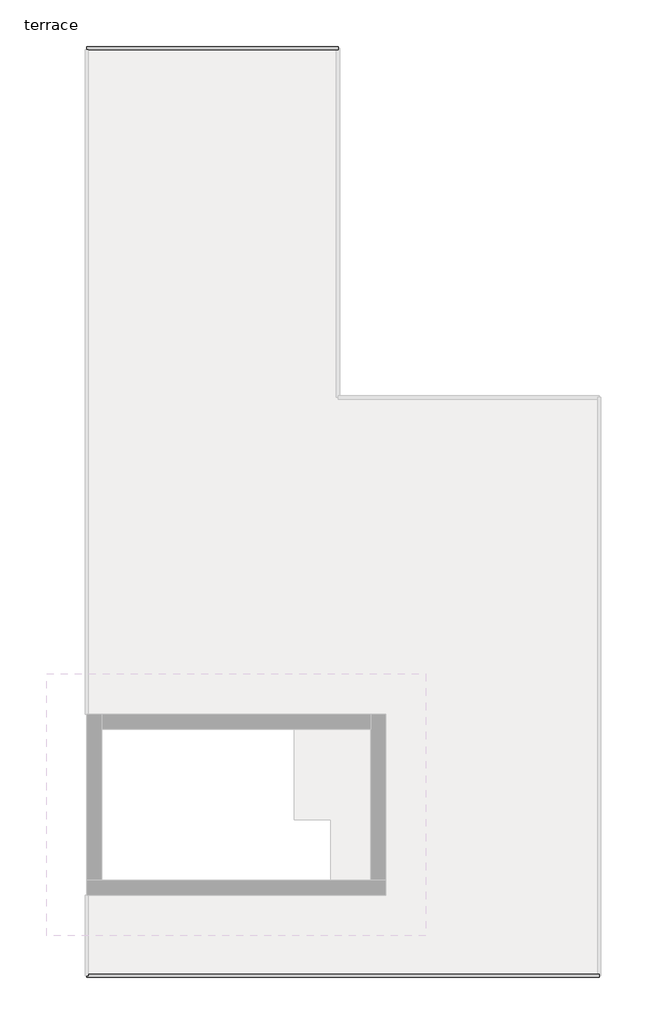
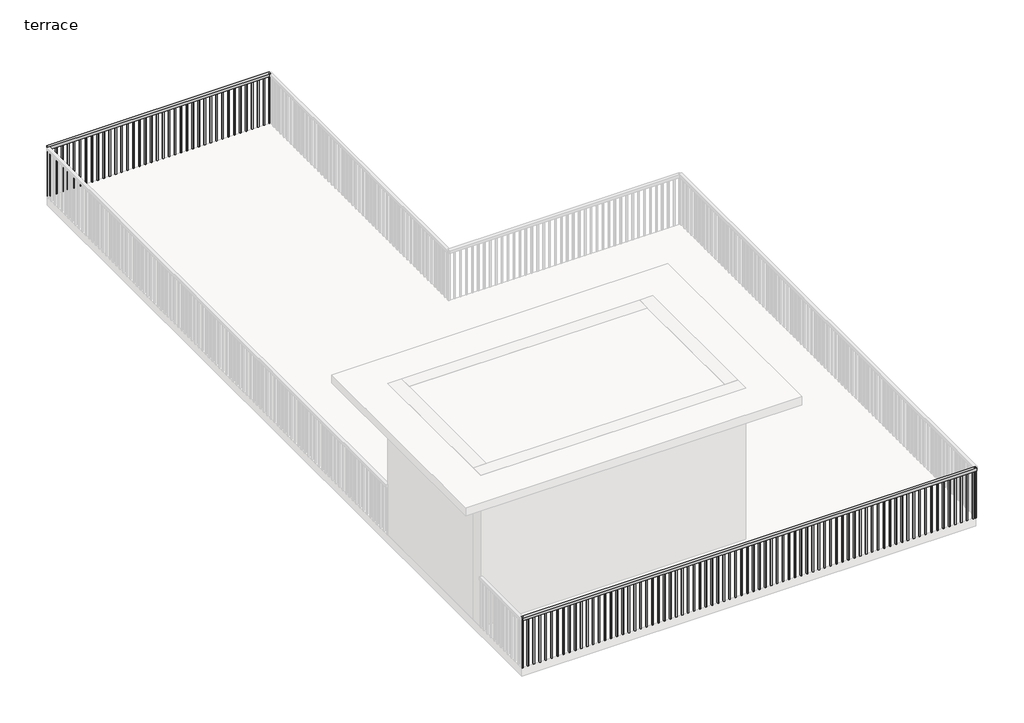
# One storey, part 2 of 4: 2 railings.
"""IFC4 building model written with IfcOpenShell, lengths in millimetres."""

from ifc_helpers import new_model, si_unit, frame, origin, place, context, project, spatial, polyline, outline, extrude, element, save

model = new_model("IFC4")

# Units and contexts
model_context = context("Model", 3, world=origin())
ifc_project = project(units=[si_unit("LENGTHUNIT", "METRE", prefix="MILLI")], contexts=[model_context])

# Site, building, storey
site = spatial("IfcSite", under=ifc_project)
building = spatial("IfcBuilding", under=site)
storey = spatial("IfcBuildingStorey", under=building, Name="terrace", Elevation=7010.4)

# Railings
placement = place(None, origin())
element("IfcRailing", 1, ObjectType="Handrail - Rectangular", at=placement, inside=storey, context=model_context, shape_type="SweptSolid", body=[
    extrude(outline(polyline([(32192.3316163, 19683.6980552), (32192.3316163, 19632.8980552), (28382.3316163, 19632.8980552), (28382.3316163, 19683.6980552), (32192.3316163, 19683.6980552)])), frame((0.0, 0.0, 7874.0), z_axis=(0.0, 0.0, 1.0), x_axis=(1.0, 0.0, 0.0)), (0.0, 0.0, 1.0), 50.8),
    extrude(outline(polyline([(28442.6566163, 19667.8230552), (28442.6566163, 19648.7730552), (28423.6066163, 19648.7730552), (28423.6066163, 19667.8230552), (28442.6566163, 19667.8230552)])), frame((0.0, 0.0, 7010.4), z_axis=(0.0, 0.0, 1.0), x_axis=(1.0, 0.0, 0.0)), (0.0, 0.0, 1.0), 863.6),
    extrude(outline(polyline([(28544.2566163, 19667.8230552), (28544.2566163, 19648.7730552), (28525.2066163, 19648.7730552), (28525.2066163, 19667.8230552), (28544.2566163, 19667.8230552)])), frame((0.0, 0.0, 7010.4), z_axis=(0.0, 0.0, 1.0), x_axis=(1.0, 0.0, 0.0)), (0.0, 0.0, 1.0), 863.6),
    extrude(outline(polyline([(28645.8566163, 19667.8230552), (28645.8566163, 19648.7730552), (28626.8066163, 19648.7730552), (28626.8066163, 19667.8230552), (28645.8566163, 19667.8230552)])), frame((0.0, 0.0, 7010.4), z_axis=(0.0, 0.0, 1.0), x_axis=(1.0, 0.0, 0.0)), (0.0, 0.0, 1.0), 863.6),
    extrude(outline(polyline([(28747.4566163, 19667.8230552), (28747.4566163, 19648.7730552), (28728.4066163, 19648.7730552), (28728.4066163, 19667.8230552), (28747.4566163, 19667.8230552)])), frame((0.0, 0.0, 7010.4), z_axis=(0.0, 0.0, 1.0), x_axis=(1.0, 0.0, 0.0)), (0.0, 0.0, 1.0), 863.6),
    extrude(outline(polyline([(28849.0566163, 19667.8230552), (28849.0566163, 19648.7730552), (28830.0066163, 19648.7730552), (28830.0066163, 19667.8230552), (28849.0566163, 19667.8230552)])), frame((0.0, 0.0, 7010.4), z_axis=(0.0, 0.0, 1.0), x_axis=(1.0, 0.0, 0.0)), (0.0, 0.0, 1.0), 863.6),
    extrude(outline(polyline([(28950.6566163, 19667.8230552), (28950.6566163, 19648.7730552), (28931.6066163, 19648.7730552), (28931.6066163, 19667.8230552), (28950.6566163, 19667.8230552)])), frame((0.0, 0.0, 7010.4), z_axis=(0.0, 0.0, 1.0), x_axis=(1.0, 0.0, 0.0)), (0.0, 0.0, 1.0), 863.6),
    extrude(outline(polyline([(29052.2566163, 19667.8230552), (29052.2566163, 19648.7730552), (29033.2066163, 19648.7730552), (29033.2066163, 19667.8230552), (29052.2566163, 19667.8230552)])), frame((0.0, 0.0, 7010.4), z_axis=(0.0, 0.0, 1.0), x_axis=(1.0, 0.0, 0.0)), (0.0, 0.0, 1.0), 863.6),
    extrude(outline(polyline([(29153.8566163, 19667.8230552), (29153.8566163, 19648.7730552), (29134.8066163, 19648.7730552), (29134.8066163, 19667.8230552), (29153.8566163, 19667.8230552)])), frame((0.0, 0.0, 7010.4), z_axis=(0.0, 0.0, 1.0), x_axis=(1.0, 0.0, 0.0)), (0.0, 0.0, 1.0), 863.6),
    extrude(outline(polyline([(29255.4566163, 19667.8230552), (29255.4566163, 19648.7730552), (29236.4066163, 19648.7730552), (29236.4066163, 19667.8230552), (29255.4566163, 19667.8230552)])), frame((0.0, 0.0, 7010.4), z_axis=(0.0, 0.0, 1.0), x_axis=(1.0, 0.0, 0.0)), (0.0, 0.0, 1.0), 863.6),
    extrude(outline(polyline([(29357.0566163, 19667.8230552), (29357.0566163, 19648.7730552), (29338.0066163, 19648.7730552), (29338.0066163, 19667.8230552), (29357.0566163, 19667.8230552)])), frame((0.0, 0.0, 7010.4), z_axis=(0.0, 0.0, 1.0), x_axis=(1.0, 0.0, 0.0)), (0.0, 0.0, 1.0), 863.6),
    extrude(outline(polyline([(29458.6566163, 19667.8230552), (29458.6566163, 19648.7730552), (29439.6066163, 19648.7730552), (29439.6066163, 19667.8230552), (29458.6566163, 19667.8230552)])), frame((0.0, 0.0, 7010.4), z_axis=(0.0, 0.0, 1.0), x_axis=(1.0, 0.0, 0.0)), (0.0, 0.0, 1.0), 863.6),
    extrude(outline(polyline([(29560.2566163, 19667.8230552), (29560.2566163, 19648.7730552), (29541.2066163, 19648.7730552), (29541.2066163, 19667.8230552), (29560.2566163, 19667.8230552)])), frame((0.0, 0.0, 7010.4), z_axis=(0.0, 0.0, 1.0), x_axis=(1.0, 0.0, 0.0)), (0.0, 0.0, 1.0), 863.6),
    extrude(outline(polyline([(29661.8566163, 19667.8230552), (29661.8566163, 19648.7730552), (29642.8066163, 19648.7730552), (29642.8066163, 19667.8230552), (29661.8566163, 19667.8230552)])), frame((0.0, 0.0, 7010.4), z_axis=(0.0, 0.0, 1.0), x_axis=(1.0, 0.0, 0.0)), (0.0, 0.0, 1.0), 863.6),
    extrude(outline(polyline([(29763.4566163, 19667.8230552), (29763.4566163, 19648.7730552), (29744.4066163, 19648.7730552), (29744.4066163, 19667.8230552), (29763.4566163, 19667.8230552)])), frame((0.0, 0.0, 7010.4), z_axis=(0.0, 0.0, 1.0), x_axis=(1.0, 0.0, 0.0)), (0.0, 0.0, 1.0), 863.6),
    extrude(outline(polyline([(29865.0566163, 19667.8230552), (29865.0566163, 19648.7730552), (29846.0066163, 19648.7730552), (29846.0066163, 19667.8230552), (29865.0566163, 19667.8230552)])), frame((0.0, 0.0, 7010.4), z_axis=(0.0, 0.0, 1.0), x_axis=(1.0, 0.0, 0.0)), (0.0, 0.0, 1.0), 863.6),
    extrude(outline(polyline([(29966.6566163, 19667.8230552), (29966.6566163, 19648.7730552), (29947.6066163, 19648.7730552), (29947.6066163, 19667.8230552), (29966.6566163, 19667.8230552)])), frame((0.0, 0.0, 7010.4), z_axis=(0.0, 0.0, 1.0), x_axis=(1.0, 0.0, 0.0)), (0.0, 0.0, 1.0), 863.6),
    extrude(outline(polyline([(30068.2566163, 19667.8230552), (30068.2566163, 19648.7730552), (30049.2066163, 19648.7730552), (30049.2066163, 19667.8230552), (30068.2566163, 19667.8230552)])), frame((0.0, 0.0, 7010.4), z_axis=(0.0, 0.0, 1.0), x_axis=(1.0, 0.0, 0.0)), (0.0, 0.0, 1.0), 863.6),
    extrude(outline(polyline([(30169.8566163, 19667.8230552), (30169.8566163, 19648.7730552), (30150.8066163, 19648.7730552), (30150.8066163, 19667.8230552), (30169.8566163, 19667.8230552)])), frame((0.0, 0.0, 7010.4), z_axis=(0.0, 0.0, 1.0), x_axis=(1.0, 0.0, 0.0)), (0.0, 0.0, 1.0), 863.6),
    extrude(outline(polyline([(30271.4566163, 19667.8230552), (30271.4566163, 19648.7730552), (30252.4066163, 19648.7730552), (30252.4066163, 19667.8230552), (30271.4566163, 19667.8230552)])), frame((0.0, 0.0, 7010.4), z_axis=(0.0, 0.0, 1.0), x_axis=(1.0, 0.0, 0.0)), (0.0, 0.0, 1.0), 863.6),
    extrude(outline(polyline([(30373.0566163, 19667.8230552), (30373.0566163, 19648.7730552), (30354.0066163, 19648.7730552), (30354.0066163, 19667.8230552), (30373.0566163, 19667.8230552)])), frame((0.0, 0.0, 7010.4), z_axis=(0.0, 0.0, 1.0), x_axis=(1.0, 0.0, 0.0)), (0.0, 0.0, 1.0), 863.6),
    extrude(outline(polyline([(30474.6566163, 19667.8230552), (30474.6566163, 19648.7730552), (30455.6066163, 19648.7730552), (30455.6066163, 19667.8230552), (30474.6566163, 19667.8230552)])), frame((0.0, 0.0, 7010.4), z_axis=(0.0, 0.0, 1.0), x_axis=(1.0, 0.0, 0.0)), (0.0, 0.0, 1.0), 863.6),
    extrude(outline(polyline([(30576.2566163, 19667.8230552), (30576.2566163, 19648.7730552), (30557.2066163, 19648.7730552), (30557.2066163, 19667.8230552), (30576.2566163, 19667.8230552)])), frame((0.0, 0.0, 7010.4), z_axis=(0.0, 0.0, 1.0), x_axis=(1.0, 0.0, 0.0)), (0.0, 0.0, 1.0), 863.6),
    extrude(outline(polyline([(30677.8566163, 19667.8230552), (30677.8566163, 19648.7730552), (30658.8066163, 19648.7730552), (30658.8066163, 19667.8230552), (30677.8566163, 19667.8230552)])), frame((0.0, 0.0, 7010.4), z_axis=(0.0, 0.0, 1.0), x_axis=(1.0, 0.0, 0.0)), (0.0, 0.0, 1.0), 863.6),
    extrude(outline(polyline([(30779.4566163, 19667.8230552), (30779.4566163, 19648.7730552), (30760.4066163, 19648.7730552), (30760.4066163, 19667.8230552), (30779.4566163, 19667.8230552)])), frame((0.0, 0.0, 7010.4), z_axis=(0.0, 0.0, 1.0), x_axis=(1.0, 0.0, 0.0)), (0.0, 0.0, 1.0), 863.6),
    extrude(outline(polyline([(30881.0566163, 19667.8230552), (30881.0566163, 19648.7730552), (30862.0066163, 19648.7730552), (30862.0066163, 19667.8230552), (30881.0566163, 19667.8230552)])), frame((0.0, 0.0, 7010.4), z_axis=(0.0, 0.0, 1.0), x_axis=(1.0, 0.0, 0.0)), (0.0, 0.0, 1.0), 863.6),
    extrude(outline(polyline([(30982.6566163, 19667.8230552), (30982.6566163, 19648.7730552), (30963.6066163, 19648.7730552), (30963.6066163, 19667.8230552), (30982.6566163, 19667.8230552)])), frame((0.0, 0.0, 7010.4), z_axis=(0.0, 0.0, 1.0), x_axis=(1.0, 0.0, 0.0)), (0.0, 0.0, 1.0), 863.6),
    extrude(outline(polyline([(31084.2566163, 19667.8230552), (31084.2566163, 19648.7730552), (31065.2066163, 19648.7730552), (31065.2066163, 19667.8230552), (31084.2566163, 19667.8230552)])), frame((0.0, 0.0, 7010.4), z_axis=(0.0, 0.0, 1.0), x_axis=(1.0, 0.0, 0.0)), (0.0, 0.0, 1.0), 863.6),
    extrude(outline(polyline([(31185.8566163, 19667.8230552), (31185.8566163, 19648.7730552), (31166.8066163, 19648.7730552), (31166.8066163, 19667.8230552), (31185.8566163, 19667.8230552)])), frame((0.0, 0.0, 7010.4), z_axis=(0.0, 0.0, 1.0), x_axis=(1.0, 0.0, 0.0)), (0.0, 0.0, 1.0), 863.6),
    extrude(outline(polyline([(31287.4566163, 19667.8230552), (31287.4566163, 19648.7730552), (31268.4066163, 19648.7730552), (31268.4066163, 19667.8230552), (31287.4566163, 19667.8230552)])), frame((0.0, 0.0, 7010.4), z_axis=(0.0, 0.0, 1.0), x_axis=(1.0, 0.0, 0.0)), (0.0, 0.0, 1.0), 863.6),
    extrude(outline(polyline([(31389.0566163, 19667.8230552), (31389.0566163, 19648.7730552), (31370.0066163, 19648.7730552), (31370.0066163, 19667.8230552), (31389.0566163, 19667.8230552)])), frame((0.0, 0.0, 7010.4), z_axis=(0.0, 0.0, 1.0), x_axis=(1.0, 0.0, 0.0)), (0.0, 0.0, 1.0), 863.6),
    extrude(outline(polyline([(31490.6566163, 19667.8230552), (31490.6566163, 19648.7730552), (31471.6066163, 19648.7730552), (31471.6066163, 19667.8230552), (31490.6566163, 19667.8230552)])), frame((0.0, 0.0, 7010.4), z_axis=(0.0, 0.0, 1.0), x_axis=(1.0, 0.0, 0.0)), (0.0, 0.0, 1.0), 863.6),
    extrude(outline(polyline([(31592.2566163, 19667.8230552), (31592.2566163, 19648.7730552), (31573.2066163, 19648.7730552), (31573.2066163, 19667.8230552), (31592.2566163, 19667.8230552)])), frame((0.0, 0.0, 7010.4), z_axis=(0.0, 0.0, 1.0), x_axis=(1.0, 0.0, 0.0)), (0.0, 0.0, 1.0), 863.6),
    extrude(outline(polyline([(31693.8566163, 19667.8230552), (31693.8566163, 19648.7730552), (31674.8066163, 19648.7730552), (31674.8066163, 19667.8230552), (31693.8566163, 19667.8230552)])), frame((0.0, 0.0, 7010.4), z_axis=(0.0, 0.0, 1.0), x_axis=(1.0, 0.0, 0.0)), (0.0, 0.0, 1.0), 863.6),
    extrude(outline(polyline([(31795.4566163, 19667.8230552), (31795.4566163, 19648.7730552), (31776.4066163, 19648.7730552), (31776.4066163, 19667.8230552), (31795.4566163, 19667.8230552)])), frame((0.0, 0.0, 7010.4), z_axis=(0.0, 0.0, 1.0), x_axis=(1.0, 0.0, 0.0)), (0.0, 0.0, 1.0), 863.6),
    extrude(outline(polyline([(31897.0566163, 19667.8230552), (31897.0566163, 19648.7730552), (31878.0066163, 19648.7730552), (31878.0066163, 19667.8230552), (31897.0566163, 19667.8230552)])), frame((0.0, 0.0, 7010.4), z_axis=(0.0, 0.0, 1.0), x_axis=(1.0, 0.0, 0.0)), (0.0, 0.0, 1.0), 863.6),
    extrude(outline(polyline([(31998.6566163, 19667.8230552), (31998.6566163, 19648.7730552), (31979.6066163, 19648.7730552), (31979.6066163, 19667.8230552), (31998.6566163, 19667.8230552)])), frame((0.0, 0.0, 7010.4), z_axis=(0.0, 0.0, 1.0), x_axis=(1.0, 0.0, 0.0)), (0.0, 0.0, 1.0), 863.6),
    extrude(outline(polyline([(32100.2566163, 19667.8230552), (32100.2566163, 19648.7730552), (32081.2066163, 19648.7730552), (32081.2066163, 19667.8230552), (32100.2566163, 19667.8230552)])), frame((0.0, 0.0, 7010.4), z_axis=(0.0, 0.0, 1.0), x_axis=(1.0, 0.0, 0.0)), (0.0, 0.0, 1.0), 863.6),
    extrude(outline(polyline([(28401.3816163, 19667.8230552), (28401.3816163, 19648.7730552), (28382.3316163, 19648.7730552), (28382.3316163, 19667.8230552), (28401.3816163, 19667.8230552)])), frame((0.0, 0.0, 7010.4), z_axis=(0.0, 0.0, 1.0), x_axis=(1.0, 0.0, 0.0)), (0.0, 0.0, 1.0), 863.6),
    extrude(outline(polyline([(32192.3316163, 19667.8230552), (32192.3316163, 19648.7730552), (32173.2816163, 19648.7730552), (32173.2816163, 19667.8230552), (32192.3316163, 19667.8230552)])), frame((0.0, 0.0, 7010.4), z_axis=(0.0, 0.0, 1.0), x_axis=(1.0, 0.0, 0.0)), (0.0, 0.0, 1.0), 863.6),
])
element("IfcRailing", 2, ObjectType="Handrail - Rectangular", at=placement, inside=storey, context=model_context, shape_type="SweptSolid", body=[
    extrude(outline(polyline([(28382.3316163, 5567.6480552), (28382.3316163, 5618.4480552), (36154.7316163, 5618.4480552), (36154.7316163, 5567.6480552), (28382.3316163, 5567.6480552)])), frame((0.0, 0.0, 7874.0), z_axis=(0.0, 0.0, 1.0), x_axis=(1.0, 0.0, 0.0)), (0.0, 0.0, 1.0), 50.8),
    extrude(outline(polyline([(36094.4066163, 5583.5230552), (36094.4066163, 5602.5730552), (36113.4566163, 5602.5730552), (36113.4566163, 5583.5230552), (36094.4066163, 5583.5230552)])), frame((0.0, 0.0, 7010.4), z_axis=(0.0, 0.0, 1.0), x_axis=(1.0, 0.0, 0.0)), (0.0, 0.0, 1.0), 863.6),
    extrude(outline(polyline([(35992.8066163, 5583.5230552), (35992.8066163, 5602.5730552), (36011.8566163, 5602.5730552), (36011.8566163, 5583.5230552), (35992.8066163, 5583.5230552)])), frame((0.0, 0.0, 7010.4), z_axis=(0.0, 0.0, 1.0), x_axis=(1.0, 0.0, 0.0)), (0.0, 0.0, 1.0), 863.6),
    extrude(outline(polyline([(35891.2066163, 5583.5230552), (35891.2066163, 5602.5730552), (35910.2566163, 5602.5730552), (35910.2566163, 5583.5230552), (35891.2066163, 5583.5230552)])), frame((0.0, 0.0, 7010.4), z_axis=(0.0, 0.0, 1.0), x_axis=(1.0, 0.0, 0.0)), (0.0, 0.0, 1.0), 863.6),
    extrude(outline(polyline([(35789.6066163, 5583.5230552), (35789.6066163, 5602.5730552), (35808.6566163, 5602.5730552), (35808.6566163, 5583.5230552), (35789.6066163, 5583.5230552)])), frame((0.0, 0.0, 7010.4), z_axis=(0.0, 0.0, 1.0), x_axis=(1.0, 0.0, 0.0)), (0.0, 0.0, 1.0), 863.6),
    extrude(outline(polyline([(35688.0066163, 5583.5230552), (35688.0066163, 5602.5730552), (35707.0566163, 5602.5730552), (35707.0566163, 5583.5230552), (35688.0066163, 5583.5230552)])), frame((0.0, 0.0, 7010.4), z_axis=(0.0, 0.0, 1.0), x_axis=(1.0, 0.0, 0.0)), (0.0, 0.0, 1.0), 863.6),
    extrude(outline(polyline([(35586.4066163, 5583.5230552), (35586.4066163, 5602.5730552), (35605.4566163, 5602.5730552), (35605.4566163, 5583.5230552), (35586.4066163, 5583.5230552)])), frame((0.0, 0.0, 7010.4), z_axis=(0.0, 0.0, 1.0), x_axis=(1.0, 0.0, 0.0)), (0.0, 0.0, 1.0), 863.6),
    extrude(outline(polyline([(35484.8066163, 5583.5230552), (35484.8066163, 5602.5730552), (35503.8566163, 5602.5730552), (35503.8566163, 5583.5230552), (35484.8066163, 5583.5230552)])), frame((0.0, 0.0, 7010.4), z_axis=(0.0, 0.0, 1.0), x_axis=(1.0, 0.0, 0.0)), (0.0, 0.0, 1.0), 863.6),
    extrude(outline(polyline([(35383.2066163, 5583.5230552), (35383.2066163, 5602.5730552), (35402.2566163, 5602.5730552), (35402.2566163, 5583.5230552), (35383.2066163, 5583.5230552)])), frame((0.0, 0.0, 7010.4), z_axis=(0.0, 0.0, 1.0), x_axis=(1.0, 0.0, 0.0)), (0.0, 0.0, 1.0), 863.6),
    extrude(outline(polyline([(35281.6066163, 5583.5230552), (35281.6066163, 5602.5730552), (35300.6566163, 5602.5730552), (35300.6566163, 5583.5230552), (35281.6066163, 5583.5230552)])), frame((0.0, 0.0, 7010.4), z_axis=(0.0, 0.0, 1.0), x_axis=(1.0, 0.0, 0.0)), (0.0, 0.0, 1.0), 863.6),
    extrude(outline(polyline([(35180.0066163, 5583.5230552), (35180.0066163, 5602.5730552), (35199.0566163, 5602.5730552), (35199.0566163, 5583.5230552), (35180.0066163, 5583.5230552)])), frame((0.0, 0.0, 7010.4), z_axis=(0.0, 0.0, 1.0), x_axis=(1.0, 0.0, 0.0)), (0.0, 0.0, 1.0), 863.6),
    extrude(outline(polyline([(35078.4066163, 5583.5230552), (35078.4066163, 5602.5730552), (35097.4566163, 5602.5730552), (35097.4566163, 5583.5230552), (35078.4066163, 5583.5230552)])), frame((0.0, 0.0, 7010.4), z_axis=(0.0, 0.0, 1.0), x_axis=(1.0, 0.0, 0.0)), (0.0, 0.0, 1.0), 863.6),
    extrude(outline(polyline([(34976.8066163, 5583.5230552), (34976.8066163, 5602.5730552), (34995.8566163, 5602.5730552), (34995.8566163, 5583.5230552), (34976.8066163, 5583.5230552)])), frame((0.0, 0.0, 7010.4), z_axis=(0.0, 0.0, 1.0), x_axis=(1.0, 0.0, 0.0)), (0.0, 0.0, 1.0), 863.6),
    extrude(outline(polyline([(34875.2066163, 5583.5230552), (34875.2066163, 5602.5730552), (34894.2566163, 5602.5730552), (34894.2566163, 5583.5230552), (34875.2066163, 5583.5230552)])), frame((0.0, 0.0, 7010.4), z_axis=(0.0, 0.0, 1.0), x_axis=(1.0, 0.0, 0.0)), (0.0, 0.0, 1.0), 863.6),
    extrude(outline(polyline([(34773.6066163, 5583.5230552), (34773.6066163, 5602.5730552), (34792.6566163, 5602.5730552), (34792.6566163, 5583.5230552), (34773.6066163, 5583.5230552)])), frame((0.0, 0.0, 7010.4), z_axis=(0.0, 0.0, 1.0), x_axis=(1.0, 0.0, 0.0)), (0.0, 0.0, 1.0), 863.6),
    extrude(outline(polyline([(34672.0066163, 5583.5230552), (34672.0066163, 5602.5730552), (34691.0566163, 5602.5730552), (34691.0566163, 5583.5230552), (34672.0066163, 5583.5230552)])), frame((0.0, 0.0, 7010.4), z_axis=(0.0, 0.0, 1.0), x_axis=(1.0, 0.0, 0.0)), (0.0, 0.0, 1.0), 863.6),
    extrude(outline(polyline([(34570.4066163, 5583.5230552), (34570.4066163, 5602.5730552), (34589.4566163, 5602.5730552), (34589.4566163, 5583.5230552), (34570.4066163, 5583.5230552)])), frame((0.0, 0.0, 7010.4), z_axis=(0.0, 0.0, 1.0), x_axis=(1.0, 0.0, 0.0)), (0.0, 0.0, 1.0), 863.6),
    extrude(outline(polyline([(34468.8066163, 5583.5230552), (34468.8066163, 5602.5730552), (34487.8566163, 5602.5730552), (34487.8566163, 5583.5230552), (34468.8066163, 5583.5230552)])), frame((0.0, 0.0, 7010.4), z_axis=(0.0, 0.0, 1.0), x_axis=(1.0, 0.0, 0.0)), (0.0, 0.0, 1.0), 863.6),
    extrude(outline(polyline([(34367.2066163, 5583.5230552), (34367.2066163, 5602.5730552), (34386.2566163, 5602.5730552), (34386.2566163, 5583.5230552), (34367.2066163, 5583.5230552)])), frame((0.0, 0.0, 7010.4), z_axis=(0.0, 0.0, 1.0), x_axis=(1.0, 0.0, 0.0)), (0.0, 0.0, 1.0), 863.6),
    extrude(outline(polyline([(34265.6066163, 5583.5230552), (34265.6066163, 5602.5730552), (34284.6566163, 5602.5730552), (34284.6566163, 5583.5230552), (34265.6066163, 5583.5230552)])), frame((0.0, 0.0, 7010.4), z_axis=(0.0, 0.0, 1.0), x_axis=(1.0, 0.0, 0.0)), (0.0, 0.0, 1.0), 863.6),
    extrude(outline(polyline([(34164.0066163, 5583.5230552), (34164.0066163, 5602.5730552), (34183.0566163, 5602.5730552), (34183.0566163, 5583.5230552), (34164.0066163, 5583.5230552)])), frame((0.0, 0.0, 7010.4), z_axis=(0.0, 0.0, 1.0), x_axis=(1.0, 0.0, 0.0)), (0.0, 0.0, 1.0), 863.6),
    extrude(outline(polyline([(34062.4066163, 5583.5230552), (34062.4066163, 5602.5730552), (34081.4566163, 5602.5730552), (34081.4566163, 5583.5230552), (34062.4066163, 5583.5230552)])), frame((0.0, 0.0, 7010.4), z_axis=(0.0, 0.0, 1.0), x_axis=(1.0, 0.0, 0.0)), (0.0, 0.0, 1.0), 863.6),
    extrude(outline(polyline([(33960.8066163, 5583.5230552), (33960.8066163, 5602.5730552), (33979.8566163, 5602.5730552), (33979.8566163, 5583.5230552), (33960.8066163, 5583.5230552)])), frame((0.0, 0.0, 7010.4), z_axis=(0.0, 0.0, 1.0), x_axis=(1.0, 0.0, 0.0)), (0.0, 0.0, 1.0), 863.6),
    extrude(outline(polyline([(33859.2066163, 5583.5230552), (33859.2066163, 5602.5730552), (33878.2566163, 5602.5730552), (33878.2566163, 5583.5230552), (33859.2066163, 5583.5230552)])), frame((0.0, 0.0, 7010.4), z_axis=(0.0, 0.0, 1.0), x_axis=(1.0, 0.0, 0.0)), (0.0, 0.0, 1.0), 863.6),
    extrude(outline(polyline([(33757.6066163, 5583.5230552), (33757.6066163, 5602.5730552), (33776.6566163, 5602.5730552), (33776.6566163, 5583.5230552), (33757.6066163, 5583.5230552)])), frame((0.0, 0.0, 7010.4), z_axis=(0.0, 0.0, 1.0), x_axis=(1.0, 0.0, 0.0)), (0.0, 0.0, 1.0), 863.6),
    extrude(outline(polyline([(33656.0066163, 5583.5230552), (33656.0066163, 5602.5730552), (33675.0566163, 5602.5730552), (33675.0566163, 5583.5230552), (33656.0066163, 5583.5230552)])), frame((0.0, 0.0, 7010.4), z_axis=(0.0, 0.0, 1.0), x_axis=(1.0, 0.0, 0.0)), (0.0, 0.0, 1.0), 863.6),
    extrude(outline(polyline([(33554.4066163, 5583.5230552), (33554.4066163, 5602.5730552), (33573.4566163, 5602.5730552), (33573.4566163, 5583.5230552), (33554.4066163, 5583.5230552)])), frame((0.0, 0.0, 7010.4), z_axis=(0.0, 0.0, 1.0), x_axis=(1.0, 0.0, 0.0)), (0.0, 0.0, 1.0), 863.6),
    extrude(outline(polyline([(33452.8066163, 5583.5230552), (33452.8066163, 5602.5730552), (33471.8566163, 5602.5730552), (33471.8566163, 5583.5230552), (33452.8066163, 5583.5230552)])), frame((0.0, 0.0, 7010.4), z_axis=(0.0, 0.0, 1.0), x_axis=(1.0, 0.0, 0.0)), (0.0, 0.0, 1.0), 863.6),
    extrude(outline(polyline([(33351.2066163, 5583.5230552), (33351.2066163, 5602.5730552), (33370.2566163, 5602.5730552), (33370.2566163, 5583.5230552), (33351.2066163, 5583.5230552)])), frame((0.0, 0.0, 7010.4), z_axis=(0.0, 0.0, 1.0), x_axis=(1.0, 0.0, 0.0)), (0.0, 0.0, 1.0), 863.6),
    extrude(outline(polyline([(33249.6066163, 5583.5230552), (33249.6066163, 5602.5730552), (33268.6566163, 5602.5730552), (33268.6566163, 5583.5230552), (33249.6066163, 5583.5230552)])), frame((0.0, 0.0, 7010.4), z_axis=(0.0, 0.0, 1.0), x_axis=(1.0, 0.0, 0.0)), (0.0, 0.0, 1.0), 863.6),
    extrude(outline(polyline([(33148.0066163, 5583.5230552), (33148.0066163, 5602.5730552), (33167.0566163, 5602.5730552), (33167.0566163, 5583.5230552), (33148.0066163, 5583.5230552)])), frame((0.0, 0.0, 7010.4), z_axis=(0.0, 0.0, 1.0), x_axis=(1.0, 0.0, 0.0)), (0.0, 0.0, 1.0), 863.6),
    extrude(outline(polyline([(33046.4066163, 5583.5230552), (33046.4066163, 5602.5730552), (33065.4566163, 5602.5730552), (33065.4566163, 5583.5230552), (33046.4066163, 5583.5230552)])), frame((0.0, 0.0, 7010.4), z_axis=(0.0, 0.0, 1.0), x_axis=(1.0, 0.0, 0.0)), (0.0, 0.0, 1.0), 863.6),
    extrude(outline(polyline([(32944.8066163, 5583.5230552), (32944.8066163, 5602.5730552), (32963.8566163, 5602.5730552), (32963.8566163, 5583.5230552), (32944.8066163, 5583.5230552)])), frame((0.0, 0.0, 7010.4), z_axis=(0.0, 0.0, 1.0), x_axis=(1.0, 0.0, 0.0)), (0.0, 0.0, 1.0), 863.6),
    extrude(outline(polyline([(32843.2066163, 5583.5230552), (32843.2066163, 5602.5730552), (32862.2566163, 5602.5730552), (32862.2566163, 5583.5230552), (32843.2066163, 5583.5230552)])), frame((0.0, 0.0, 7010.4), z_axis=(0.0, 0.0, 1.0), x_axis=(1.0, 0.0, 0.0)), (0.0, 0.0, 1.0), 863.6),
    extrude(outline(polyline([(32741.6066163, 5583.5230552), (32741.6066163, 5602.5730552), (32760.6566163, 5602.5730552), (32760.6566163, 5583.5230552), (32741.6066163, 5583.5230552)])), frame((0.0, 0.0, 7010.4), z_axis=(0.0, 0.0, 1.0), x_axis=(1.0, 0.0, 0.0)), (0.0, 0.0, 1.0), 863.6),
    extrude(outline(polyline([(32640.0066163, 5583.5230552), (32640.0066163, 5602.5730552), (32659.0566163, 5602.5730552), (32659.0566163, 5583.5230552), (32640.0066163, 5583.5230552)])), frame((0.0, 0.0, 7010.4), z_axis=(0.0, 0.0, 1.0), x_axis=(1.0, 0.0, 0.0)), (0.0, 0.0, 1.0), 863.6),
    extrude(outline(polyline([(32538.4066163, 5583.5230552), (32538.4066163, 5602.5730552), (32557.4566163, 5602.5730552), (32557.4566163, 5583.5230552), (32538.4066163, 5583.5230552)])), frame((0.0, 0.0, 7010.4), z_axis=(0.0, 0.0, 1.0), x_axis=(1.0, 0.0, 0.0)), (0.0, 0.0, 1.0), 863.6),
    extrude(outline(polyline([(32436.8066163, 5583.5230552), (32436.8066163, 5602.5730552), (32455.8566163, 5602.5730552), (32455.8566163, 5583.5230552), (32436.8066163, 5583.5230552)])), frame((0.0, 0.0, 7010.4), z_axis=(0.0, 0.0, 1.0), x_axis=(1.0, 0.0, 0.0)), (0.0, 0.0, 1.0), 863.6),
    extrude(outline(polyline([(32335.2066163, 5583.5230552), (32335.2066163, 5602.5730552), (32354.2566163, 5602.5730552), (32354.2566163, 5583.5230552), (32335.2066163, 5583.5230552)])), frame((0.0, 0.0, 7010.4), z_axis=(0.0, 0.0, 1.0), x_axis=(1.0, 0.0, 0.0)), (0.0, 0.0, 1.0), 863.6),
    extrude(outline(polyline([(32233.6066163, 5583.5230552), (32233.6066163, 5602.5730552), (32252.6566163, 5602.5730552), (32252.6566163, 5583.5230552), (32233.6066163, 5583.5230552)])), frame((0.0, 0.0, 7010.4), z_axis=(0.0, 0.0, 1.0), x_axis=(1.0, 0.0, 0.0)), (0.0, 0.0, 1.0), 863.6),
    extrude(outline(polyline([(32132.0066163, 5583.5230552), (32132.0066163, 5602.5730552), (32151.0566163, 5602.5730552), (32151.0566163, 5583.5230552), (32132.0066163, 5583.5230552)])), frame((0.0, 0.0, 7010.4), z_axis=(0.0, 0.0, 1.0), x_axis=(1.0, 0.0, 0.0)), (0.0, 0.0, 1.0), 863.6),
    extrude(outline(polyline([(32030.4066163, 5583.5230552), (32030.4066163, 5602.5730552), (32049.4566163, 5602.5730552), (32049.4566163, 5583.5230552), (32030.4066163, 5583.5230552)])), frame((0.0, 0.0, 7010.4), z_axis=(0.0, 0.0, 1.0), x_axis=(1.0, 0.0, 0.0)), (0.0, 0.0, 1.0), 863.6),
    extrude(outline(polyline([(31928.8066163, 5583.5230552), (31928.8066163, 5602.5730552), (31947.8566163, 5602.5730552), (31947.8566163, 5583.5230552), (31928.8066163, 5583.5230552)])), frame((0.0, 0.0, 7010.4), z_axis=(0.0, 0.0, 1.0), x_axis=(1.0, 0.0, 0.0)), (0.0, 0.0, 1.0), 863.6),
    extrude(outline(polyline([(31827.2066163, 5583.5230552), (31827.2066163, 5602.5730552), (31846.2566163, 5602.5730552), (31846.2566163, 5583.5230552), (31827.2066163, 5583.5230552)])), frame((0.0, 0.0, 7010.4), z_axis=(0.0, 0.0, 1.0), x_axis=(1.0, 0.0, 0.0)), (0.0, 0.0, 1.0), 863.6),
    extrude(outline(polyline([(31725.6066163, 5583.5230552), (31725.6066163, 5602.5730552), (31744.6566163, 5602.5730552), (31744.6566163, 5583.5230552), (31725.6066163, 5583.5230552)])), frame((0.0, 0.0, 7010.4), z_axis=(0.0, 0.0, 1.0), x_axis=(1.0, 0.0, 0.0)), (0.0, 0.0, 1.0), 863.6),
    extrude(outline(polyline([(31624.0066163, 5583.5230552), (31624.0066163, 5602.5730552), (31643.0566163, 5602.5730552), (31643.0566163, 5583.5230552), (31624.0066163, 5583.5230552)])), frame((0.0, 0.0, 7010.4), z_axis=(0.0, 0.0, 1.0), x_axis=(1.0, 0.0, 0.0)), (0.0, 0.0, 1.0), 863.6),
    extrude(outline(polyline([(31522.4066163, 5583.5230552), (31522.4066163, 5602.5730552), (31541.4566163, 5602.5730552), (31541.4566163, 5583.5230552), (31522.4066163, 5583.5230552)])), frame((0.0, 0.0, 7010.4), z_axis=(0.0, 0.0, 1.0), x_axis=(1.0, 0.0, 0.0)), (0.0, 0.0, 1.0), 863.6),
    extrude(outline(polyline([(31420.8066163, 5583.5230552), (31420.8066163, 5602.5730552), (31439.8566163, 5602.5730552), (31439.8566163, 5583.5230552), (31420.8066163, 5583.5230552)])), frame((0.0, 0.0, 7010.4), z_axis=(0.0, 0.0, 1.0), x_axis=(1.0, 0.0, 0.0)), (0.0, 0.0, 1.0), 863.6),
    extrude(outline(polyline([(31319.2066163, 5583.5230552), (31319.2066163, 5602.5730552), (31338.2566163, 5602.5730552), (31338.2566163, 5583.5230552), (31319.2066163, 5583.5230552)])), frame((0.0, 0.0, 7010.4), z_axis=(0.0, 0.0, 1.0), x_axis=(1.0, 0.0, 0.0)), (0.0, 0.0, 1.0), 863.6),
    extrude(outline(polyline([(31217.6066163, 5583.5230552), (31217.6066163, 5602.5730552), (31236.6566163, 5602.5730552), (31236.6566163, 5583.5230552), (31217.6066163, 5583.5230552)])), frame((0.0, 0.0, 7010.4), z_axis=(0.0, 0.0, 1.0), x_axis=(1.0, 0.0, 0.0)), (0.0, 0.0, 1.0), 863.6),
    extrude(outline(polyline([(31116.0066163, 5583.5230552), (31116.0066163, 5602.5730552), (31135.0566163, 5602.5730552), (31135.0566163, 5583.5230552), (31116.0066163, 5583.5230552)])), frame((0.0, 0.0, 7010.4), z_axis=(0.0, 0.0, 1.0), x_axis=(1.0, 0.0, 0.0)), (0.0, 0.0, 1.0), 863.6),
    extrude(outline(polyline([(31014.4066163, 5583.5230552), (31014.4066163, 5602.5730552), (31033.4566163, 5602.5730552), (31033.4566163, 5583.5230552), (31014.4066163, 5583.5230552)])), frame((0.0, 0.0, 7010.4), z_axis=(0.0, 0.0, 1.0), x_axis=(1.0, 0.0, 0.0)), (0.0, 0.0, 1.0), 863.6),
    extrude(outline(polyline([(30912.8066163, 5583.5230552), (30912.8066163, 5602.5730552), (30931.8566163, 5602.5730552), (30931.8566163, 5583.5230552), (30912.8066163, 5583.5230552)])), frame((0.0, 0.0, 7010.4), z_axis=(0.0, 0.0, 1.0), x_axis=(1.0, 0.0, 0.0)), (0.0, 0.0, 1.0), 863.6),
    extrude(outline(polyline([(30811.2066163, 5583.5230552), (30811.2066163, 5602.5730552), (30830.2566163, 5602.5730552), (30830.2566163, 5583.5230552), (30811.2066163, 5583.5230552)])), frame((0.0, 0.0, 7010.4), z_axis=(0.0, 0.0, 1.0), x_axis=(1.0, 0.0, 0.0)), (0.0, 0.0, 1.0), 863.6),
    extrude(outline(polyline([(30709.6066163, 5583.5230552), (30709.6066163, 5602.5730552), (30728.6566163, 5602.5730552), (30728.6566163, 5583.5230552), (30709.6066163, 5583.5230552)])), frame((0.0, 0.0, 7010.4), z_axis=(0.0, 0.0, 1.0), x_axis=(1.0, 0.0, 0.0)), (0.0, 0.0, 1.0), 863.6),
    extrude(outline(polyline([(30608.0066163, 5583.5230552), (30608.0066163, 5602.5730552), (30627.0566163, 5602.5730552), (30627.0566163, 5583.5230552), (30608.0066163, 5583.5230552)])), frame((0.0, 0.0, 7010.4), z_axis=(0.0, 0.0, 1.0), x_axis=(1.0, 0.0, 0.0)), (0.0, 0.0, 1.0), 863.6),
    extrude(outline(polyline([(30506.4066163, 5583.5230552), (30506.4066163, 5602.5730552), (30525.4566163, 5602.5730552), (30525.4566163, 5583.5230552), (30506.4066163, 5583.5230552)])), frame((0.0, 0.0, 7010.4), z_axis=(0.0, 0.0, 1.0), x_axis=(1.0, 0.0, 0.0)), (0.0, 0.0, 1.0), 863.6),
    extrude(outline(polyline([(30404.8066163, 5583.5230552), (30404.8066163, 5602.5730552), (30423.8566163, 5602.5730552), (30423.8566163, 5583.5230552), (30404.8066163, 5583.5230552)])), frame((0.0, 0.0, 7010.4), z_axis=(0.0, 0.0, 1.0), x_axis=(1.0, 0.0, 0.0)), (0.0, 0.0, 1.0), 863.6),
    extrude(outline(polyline([(30303.2066163, 5583.5230552), (30303.2066163, 5602.5730552), (30322.2566163, 5602.5730552), (30322.2566163, 5583.5230552), (30303.2066163, 5583.5230552)])), frame((0.0, 0.0, 7010.4), z_axis=(0.0, 0.0, 1.0), x_axis=(1.0, 0.0, 0.0)), (0.0, 0.0, 1.0), 863.6),
    extrude(outline(polyline([(30201.6066163, 5583.5230552), (30201.6066163, 5602.5730552), (30220.6566163, 5602.5730552), (30220.6566163, 5583.5230552), (30201.6066163, 5583.5230552)])), frame((0.0, 0.0, 7010.4), z_axis=(0.0, 0.0, 1.0), x_axis=(1.0, 0.0, 0.0)), (0.0, 0.0, 1.0), 863.6),
    extrude(outline(polyline([(30100.0066163, 5583.5230552), (30100.0066163, 5602.5730552), (30119.0566163, 5602.5730552), (30119.0566163, 5583.5230552), (30100.0066163, 5583.5230552)])), frame((0.0, 0.0, 7010.4), z_axis=(0.0, 0.0, 1.0), x_axis=(1.0, 0.0, 0.0)), (0.0, 0.0, 1.0), 863.6),
    extrude(outline(polyline([(29998.4066163, 5583.5230552), (29998.4066163, 5602.5730552), (30017.4566163, 5602.5730552), (30017.4566163, 5583.5230552), (29998.4066163, 5583.5230552)])), frame((0.0, 0.0, 7010.4), z_axis=(0.0, 0.0, 1.0), x_axis=(1.0, 0.0, 0.0)), (0.0, 0.0, 1.0), 863.6),
    extrude(outline(polyline([(29896.8066163, 5583.5230552), (29896.8066163, 5602.5730552), (29915.8566163, 5602.5730552), (29915.8566163, 5583.5230552), (29896.8066163, 5583.5230552)])), frame((0.0, 0.0, 7010.4), z_axis=(0.0, 0.0, 1.0), x_axis=(1.0, 0.0, 0.0)), (0.0, 0.0, 1.0), 863.6),
    extrude(outline(polyline([(29795.2066163, 5583.5230552), (29795.2066163, 5602.5730552), (29814.2566163, 5602.5730552), (29814.2566163, 5583.5230552), (29795.2066163, 5583.5230552)])), frame((0.0, 0.0, 7010.4), z_axis=(0.0, 0.0, 1.0), x_axis=(1.0, 0.0, 0.0)), (0.0, 0.0, 1.0), 863.6),
    extrude(outline(polyline([(29693.6066163, 5583.5230552), (29693.6066163, 5602.5730552), (29712.6566163, 5602.5730552), (29712.6566163, 5583.5230552), (29693.6066163, 5583.5230552)])), frame((0.0, 0.0, 7010.4), z_axis=(0.0, 0.0, 1.0), x_axis=(1.0, 0.0, 0.0)), (0.0, 0.0, 1.0), 863.6),
    extrude(outline(polyline([(29592.0066163, 5583.5230552), (29592.0066163, 5602.5730552), (29611.0566163, 5602.5730552), (29611.0566163, 5583.5230552), (29592.0066163, 5583.5230552)])), frame((0.0, 0.0, 7010.4), z_axis=(0.0, 0.0, 1.0), x_axis=(1.0, 0.0, 0.0)), (0.0, 0.0, 1.0), 863.6),
    extrude(outline(polyline([(29490.4066163, 5583.5230552), (29490.4066163, 5602.5730552), (29509.4566163, 5602.5730552), (29509.4566163, 5583.5230552), (29490.4066163, 5583.5230552)])), frame((0.0, 0.0, 7010.4), z_axis=(0.0, 0.0, 1.0), x_axis=(1.0, 0.0, 0.0)), (0.0, 0.0, 1.0), 863.6),
    extrude(outline(polyline([(29388.8066163, 5583.5230552), (29388.8066163, 5602.5730552), (29407.8566163, 5602.5730552), (29407.8566163, 5583.5230552), (29388.8066163, 5583.5230552)])), frame((0.0, 0.0, 7010.4), z_axis=(0.0, 0.0, 1.0), x_axis=(1.0, 0.0, 0.0)), (0.0, 0.0, 1.0), 863.6),
    extrude(outline(polyline([(29287.2066163, 5583.5230552), (29287.2066163, 5602.5730552), (29306.2566163, 5602.5730552), (29306.2566163, 5583.5230552), (29287.2066163, 5583.5230552)])), frame((0.0, 0.0, 7010.4), z_axis=(0.0, 0.0, 1.0), x_axis=(1.0, 0.0, 0.0)), (0.0, 0.0, 1.0), 863.6),
    extrude(outline(polyline([(29185.6066163, 5583.5230552), (29185.6066163, 5602.5730552), (29204.6566163, 5602.5730552), (29204.6566163, 5583.5230552), (29185.6066163, 5583.5230552)])), frame((0.0, 0.0, 7010.4), z_axis=(0.0, 0.0, 1.0), x_axis=(1.0, 0.0, 0.0)), (0.0, 0.0, 1.0), 863.6),
    extrude(outline(polyline([(29084.0066163, 5583.5230552), (29084.0066163, 5602.5730552), (29103.0566163, 5602.5730552), (29103.0566163, 5583.5230552), (29084.0066163, 5583.5230552)])), frame((0.0, 0.0, 7010.4), z_axis=(0.0, 0.0, 1.0), x_axis=(1.0, 0.0, 0.0)), (0.0, 0.0, 1.0), 863.6),
    extrude(outline(polyline([(28982.4066163, 5583.5230552), (28982.4066163, 5602.5730552), (29001.4566163, 5602.5730552), (29001.4566163, 5583.5230552), (28982.4066163, 5583.5230552)])), frame((0.0, 0.0, 7010.4), z_axis=(0.0, 0.0, 1.0), x_axis=(1.0, 0.0, 0.0)), (0.0, 0.0, 1.0), 863.6),
    extrude(outline(polyline([(28880.8066163, 5583.5230552), (28880.8066163, 5602.5730552), (28899.8566163, 5602.5730552), (28899.8566163, 5583.5230552), (28880.8066163, 5583.5230552)])), frame((0.0, 0.0, 7010.4), z_axis=(0.0, 0.0, 1.0), x_axis=(1.0, 0.0, 0.0)), (0.0, 0.0, 1.0), 863.6),
    extrude(outline(polyline([(28779.2066163, 5583.5230552), (28779.2066163, 5602.5730552), (28798.2566163, 5602.5730552), (28798.2566163, 5583.5230552), (28779.2066163, 5583.5230552)])), frame((0.0, 0.0, 7010.4), z_axis=(0.0, 0.0, 1.0), x_axis=(1.0, 0.0, 0.0)), (0.0, 0.0, 1.0), 863.6),
    extrude(outline(polyline([(28677.6066163, 5583.5230552), (28677.6066163, 5602.5730552), (28696.6566163, 5602.5730552), (28696.6566163, 5583.5230552), (28677.6066163, 5583.5230552)])), frame((0.0, 0.0, 7010.4), z_axis=(0.0, 0.0, 1.0), x_axis=(1.0, 0.0, 0.0)), (0.0, 0.0, 1.0), 863.6),
    extrude(outline(polyline([(28576.0066163, 5583.5230552), (28576.0066163, 5602.5730552), (28595.0566163, 5602.5730552), (28595.0566163, 5583.5230552), (28576.0066163, 5583.5230552)])), frame((0.0, 0.0, 7010.4), z_axis=(0.0, 0.0, 1.0), x_axis=(1.0, 0.0, 0.0)), (0.0, 0.0, 1.0), 863.6),
    extrude(outline(polyline([(28474.4066163, 5583.5230552), (28474.4066163, 5602.5730552), (28493.4566163, 5602.5730552), (28493.4566163, 5583.5230552), (28474.4066163, 5583.5230552)])), frame((0.0, 0.0, 7010.4), z_axis=(0.0, 0.0, 1.0), x_axis=(1.0, 0.0, 0.0)), (0.0, 0.0, 1.0), 863.6),
    extrude(outline(polyline([(36135.6816163, 5583.5230552), (36135.6816163, 5602.5730552), (36154.7316163, 5602.5730552), (36154.7316163, 5583.5230552), (36135.6816163, 5583.5230552)])), frame((0.0, 0.0, 7010.4), z_axis=(0.0, 0.0, 1.0), x_axis=(1.0, 0.0, 0.0)), (0.0, 0.0, 1.0), 863.6),
    extrude(outline(polyline([(28382.3316163, 5583.5230552), (28382.3316163, 5602.5730552), (28401.3816163, 5602.5730552), (28401.3816163, 5583.5230552), (28382.3316163, 5583.5230552)])), frame((0.0, 0.0, 7010.4), z_axis=(0.0, 0.0, 1.0), x_axis=(1.0, 0.0, 0.0)), (0.0, 0.0, 1.0), 863.6),
])

save(model, "model.ifc")

# Revit data of these elements
# Type "Handrail - Rectangular"
#   Assembly Code = "C2010400"
#   built-in parameter 1008612 = 0.0416667 (stored number, unit not read)
#   built-in parameter 1008611 = 0.0416667 (stored number, unit not read)
#   built-in parameter 1008609 = 0.333333 (stored number, unit not read)
#   built-in parameter 1008604 = 0.166667 (stored number, unit not read)
#   built-in parameter 1008603 = 0.166667 (stored number, unit not read)
#   Railing Height = 3' - 0"
#   built-in parameter 1008630 = 2
#   built-in parameter 1008610 = 2
#   built-in parameter 1008618 = Baluster - Square : 3/4"
# Elements 1, 2 (IfcRailing, "Handrail - Rectangular")
#   Phase Created = New Construction
